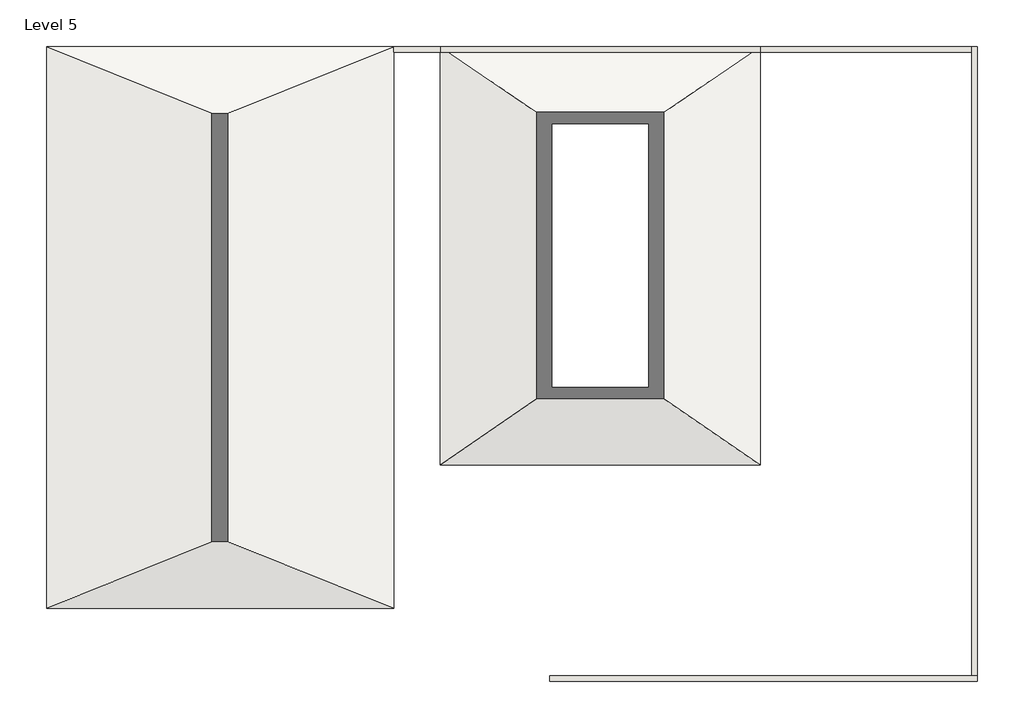
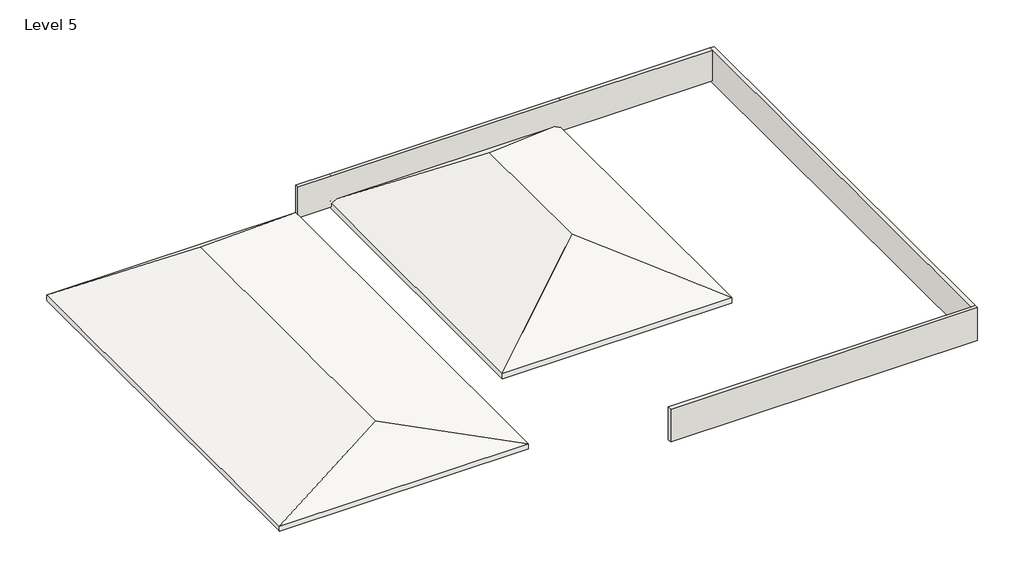
# One storey: 3 walls, 2 roofs.
"""IFC4 building model written with IfcOpenShell, lengths in millimetres."""

from ifc_helpers import new_model, si_unit, origin, place, context, project, spatial, faceted_brep, element, save

model = new_model("IFC4")

# Units and contexts
model_context = context("Model", 3, world=origin())
ifc_project = project(units=[si_unit("LENGTHUNIT", "METRE", prefix="MILLI")], contexts=[model_context])

# Site, building, storey
site = spatial("IfcSite", under=ifc_project)
building = spatial("IfcBuilding", under=site)
storey = spatial("IfcBuildingStorey", under=building, Name="Level 5", Elevation=7620.0)

# Roofs
placement = place(None, origin())
element("IfcRoof", 1, ObjectType="6\" roof", at=placement, inside=storey, context=model_context, shape_type="Brep", body=[
    faceted_brep([(-10622.0352284, -3115.6899642, 7620.0), (-7001.1418145, -1658.6194616, 8712.802877), (-3380.2484006, -3115.6899642, 7620.0), (-7001.1418145, 7072.1949279, 8712.802877), (-3380.2484006, 8529.2654305, 7620.0), (-10622.0352284, 8529.2654305, 7620.0), (-10622.0352284, -3157.4372669, 7779.189523), (-3380.2484006, -3157.4372669, 7779.189523), (-7001.1418145, -1700.3667642, 8871.9924), (-3380.2484006, 8571.0127331, 7779.189523), (-7001.1418145, 7113.9422305, 8871.9924), (-10622.0352284, 8571.0127331, 7779.189523), (-3380.2484006, -3157.4372669, 7620.0), (-10622.0352284, -3157.4372669, 7620.0), (-3380.2484006, 8571.0127331, 7620.0), (-10622.0352284, 8571.0127331, 7620.0)], [[[0, 1, 2]], [[2, 1, 3, 4]], [[4, 3, 5]], [[1, 0, 5, 3]], [[6, 7, 8]], [[7, 9, 10, 8]], [[9, 11, 10]], [[6, 8, 10, 11]], [[12, 7, 6, 13]], [[14, 9, 7, 12, 2, 4]], [[15, 11, 9, 14]], [[13, 6, 11, 15, 5, 0]], [[13, 0, 2, 12]], [[5, 15, 14, 4]]]),
])
element("IfcRoof", 2, ObjectType="Generic - 12\"", at=placement, inside=storey, context=model_context, shape_type="Brep", body=[
    faceted_brep([(4260.3793226, 8545.6327528, 7620.0), (927.6434192, 6254.4735848, 9338.369376), (-2405.0924842, 8545.6327528, 7620.0), (927.6434192, 2156.3018814, 9338.369376), (-2405.0924842, -134.8572866, 7620.0), (4260.3793226, -134.8572866, 7620.0), (4260.3793226, 8571.0127331, 7791.4650148), (-2405.0924842, 8571.0127331, 7791.4650148), (927.6434192, 6279.8535651, 9509.8343908), (-2405.0924842, -160.2372669, 7791.4650148), (927.6434192, 2130.9219011, 9509.8343908), (4260.3793226, -160.2372669, 7791.4650148), (-2405.0924842, 8571.0127331, 7620.0), (4260.3793226, 8571.0127331, 7620.0), (-2405.0924842, -160.2372669, 7620.0), (4260.3793226, -160.2372669, 7620.0)], [[[0, 1, 2]], [[2, 1, 3, 4]], [[4, 3, 5]], [[1, 0, 5, 3]], [[6, 7, 8]], [[7, 9, 10, 8]], [[9, 11, 10]], [[6, 8, 10, 11]], [[12, 7, 6, 13]], [[14, 9, 7, 12, 2, 4]], [[15, 11, 9, 14]], [[13, 6, 11, 15, 5, 0]], [[13, 0, 2, 12]], [[5, 15, 14, 4]]]),
])

# Walls
element("IfcWall", 3, ObjectType="4.5\" wall", at=placement, inside=storey, context=model_context, shape_type="Brep", body=[
    faceted_brep([(8795.3412199, -4567.1372669, 7620.0), (8681.0412199, -4567.1372669, 7620.0), (-129.0484006, -4567.1372669, 7620.0), (-129.0484006, -4567.1372669, 8627.7427173), (8681.0412199, -4567.1372669, 8627.7427173), (8795.3412199, -4567.1372669, 8627.7427173), (8795.3412199, -4681.4372669, 7620.0), (8795.3412199, -4681.4372669, 8627.7427173), (-129.0484006, -4681.4372669, 8627.7427173), (-129.0484006, -4681.4372669, 7620.0)], [[[0, 1, 2, 3, 4, 5]], [[6, 7, 8, 9]], [[2, 1, 0, 6, 9]], [[3, 2, 9, 8]], [[5, 4, 3, 8, 7]], [[0, 5, 7, 6]]]),
])
element("IfcWall", 4, ObjectType="4.5\" wall", at=placement, inside=storey, context=model_context, shape_type="Brep", body=[
    faceted_brep([(8681.0412199, 8571.0127331, 7620.0), (8681.0412199, 8545.6327528, 7620.0), (8681.0412199, -4567.1372669, 7620.0), (8681.0412199, -4567.1372669, 8627.7427173), (8681.0412199, 8456.7127331, 8627.7427173), (8681.0412199, 8571.0127331, 8627.7427173), (8795.3412199, 8571.0127331, 7620.0), (8795.3412199, 8571.0127331, 8627.7427173), (8795.3412199, -4567.1372669, 8627.7427173), (8795.3412199, -4567.1372669, 7620.0)], [[[0, 1, 2, 3, 4, 5]], [[6, 7, 8, 9]], [[2, 1, 0, 6, 9]], [[5, 4, 3, 8, 7]], [[0, 5, 7, 6]], [[3, 2, 9, 8]]]),
])
element("IfcWall", 5, ObjectType="4.5\" wall", at=placement, inside=storey, context=model_context, shape_type="Brep", body=[
    faceted_brep([(8681.0412199, 8571.0127331, 7620.0), (-3380.2484006, 8571.0127331, 7620.0), (-3380.2484006, 8571.0127331, 8627.7427173), (-2405.0924842, 8571.0127331, 8627.7427173), (4260.3793226, 8571.0127331, 8627.7427173), (8681.0412199, 8571.0127331, 8627.7427173), (-2405.0924842, 8456.7127331, 8627.7427173), (-3380.2484006, 8456.7127331, 8627.7427173), (-3380.2484006, 8456.7127331, 7686.6900148), (8681.0412199, 8456.7127331, 7686.6900148), (8681.0412199, 8456.7127331, 8627.7427173), (4260.3793226, 8456.7127331, 8627.7427173), (8681.0412199, 8545.6327528, 7620.0), (-3380.2484006, 8545.6327528, 7620.0)], [[[0, 1, 2, 3, 4, 5]], [[6, 7, 8, 9, 10, 11]], [[1, 0, 12, 13]], [[2, 1, 13, 8, 7]], [[0, 5, 10, 9, 12]], [[2, 7, 6, 3]], [[3, 6, 11, 4]], [[10, 5, 4, 11]], [[9, 8, 13, 12]]]),
])

save(model, "model.ifc")

# Revit data of these elements
# Type "6\" roof"
#   Assembly Code = "B1020"
#   Layers, outside or top first: 0' - 6" "roof" (function 1)
# Type "Generic - 12\""
#   Assembly Code = "B1020"
#   Layers, outside or top first: 0' - 6" "roof" (function 1)
# Type "4.5\" wall"
#   Assembly Code = "B2010"
#   Layers, outside or top first: 0' - 4 1/2" "Wall" (function 1)
# Element 1 (IfcRoof, "6\" roof")
#   built-in parameter 1001705 = 29.1076 (stored number, unit not read)
#   built-in parameter 1001710 = 33615
#   Phase Created = New Construction
#   Materials on its faces: "roof"
# Element 2 (IfcRoof, "Generic - 12\"")
#   built-in parameter 1001705 = 31.2002 (stored number, unit not read)
#   built-in parameter 1001710 = 33615
#   Phase Created = New Construction
#   Materials on its faces: "roof"
# Elements 3, 4, 5 (IfcWall, "4.5\" wall")
#   Top Offset = 0' - 0"
#   Base Offset = 0' - 0"
#   Unconnected Height = 3' - 3.67491"
#   wall height = 3' - 3.67491"
#   Phase Created = New Construction
#   Base Constraint = Level 5
#   Materials on its faces: "Wall"
# Materials
#   "roof": class "Generic", colour RGB 120 120 120, transparency 0, Cost = 0
#   "Wall": class "Generic", colour RGB 120 120 120, transparency 0, Cost = 0
